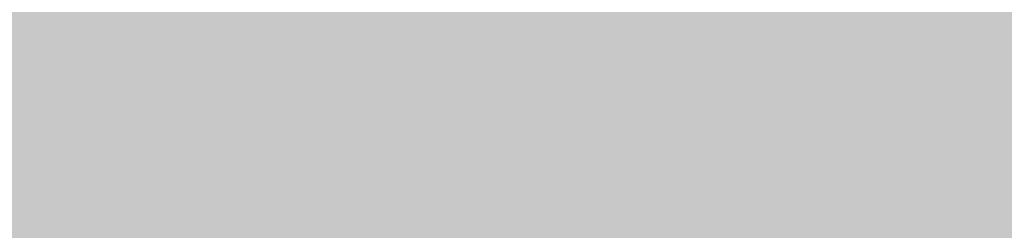
# Model space of a CAD drawing. Units: millimetres. Extents: x -22994 to 29398, y -19990 to 20176.
# Tile 73 of 135: x 226.355 to 227.437, y 83.564 to 83.796. Entities that reach past the tile are written whole.
import ezdxf
from ezdxf import colors
from ezdxf.entities.mleader import LeaderData, LeaderLine
from ezdxf.math import Vec2, Vec3

# ---------------------------------------------------------------- set-up
doc = ezdxf.new("R2010")
doc.units = ezdxf.units.MM
doc.header["$MEASUREMENT"] = 0
for name, color, linetype, lineweight in [('M-ANNO-TEXT', 7, 'Continuous', 25), ('M-DIMS', 2, 'Continuous', 18), ('M-EQPM-PATT', 7, 'Continuous', 18)]:
    doc.layers.add(name, color=color, linetype=linetype, lineweight=lineweight)
doc.styles.get("Standard").update_dxf_attribs({"font": 'arial.ttf'})
doc.dimstyles.get("Standard").update_dxf_attribs({"dimtxt": 0.18, "dimasz": 10000, "dimexe": 0.18, "dimexo": 0.0625, "dimgap": 0.09, "dimtad": 0, "dimtih": 1, "dimtoh": 1, "dimdec": 0, "dimzin": 0, "dimdsep": 46, "dimtxsty": 'Standard', "dimcen": 0.09, "dimadec": 0, "dimazin": 0, "dimtfac": 1, "dimtdec": 0, "dimtofl": 0, "dimtmove": 0, "dimatfit": 3, "dimfxl": 1, "dimtolj": 1, "dimtzin": 0, "dimlwd": 30, "dimarcsym": 0})

# ---------------------------------------------------------------- blocks, each defined once
blk = doc.blocks.new('*D2')
at = {"layer": 'Defpoints', "color": 0, "transparency": 16777216}
for p in [(6.6773, 10.2713), (290.852, 10.2713), (290.852, -5.0787)]:
    blk.add_point(p, dxfattribs=at)
at = {"layer": 'M-DIMS', "color": 0, "lineweight": -2, "transparency": 16777216}
for p, q in [((6.6773, 10.2088), (6.6773, -5.2587)), ((290.852, 10.2088), (290.852, -5.2587))]:
    blk.add_line(p, q, dxfattribs=at)
at = {"layer": 'M-DIMS', "color": 0, "lineweight": 30, "transparency": 16777216}
for p, q in [((-9993.3227, -5.0787), (-19993.3227, -5.0787)), ((10290.852, -5.0787), (20290.852, -5.0787))]:
    blk.add_line(p, q, dxfattribs=at)
at = {"layer": 'M-DIMS', "color": 0, "transparency": 16777216}
for points in [[(-9993.3227, 1661.5879), (-9993.3227, -1671.7454), (6.6773, -5.0787)], [(10290.852, 1661.5879), (10290.852, -1671.7454), (290.852, -5.0787)]]:
    blk.add_solid(points, dxfattribs=at)
at = {"layer": 'M-DIMS', "color": 0, "transparency": 16777216, "insert": (148.7647, -5.0787), "char_height": 0.18, "attachment_point": 5}
blk.add_mtext('\\A1;284.2', dxfattribs=at)
blk = doc.blocks.new('*D3')
at = {"layer": 'Defpoints', "color": 0, "transparency": 16777216}
for p in [(110.2647, 204.1654), (110.2647, 176.3662), (95.8327, 127.967)]:
    blk.add_point(p, dxfattribs=at)
at = {"layer": 'M-DIMS', "color": 0, "lineweight": -2, "transparency": 16777216}
for p, q in [((95.8327, 128.0295), (95.8327, 204.3454)), ((110.2647, 176.4287), (110.2647, 204.3454))]:
    blk.add_line(p, q, dxfattribs=at)
at = {"layer": 'M-DIMS', "color": 0, "lineweight": 30, "transparency": 16777216}
for p, q in [((-9904.1673, 204.1654), (-19904.1673, 204.1654)), ((10110.2647, 204.1654), (20110.2647, 204.1654))]:
    blk.add_line(p, q, dxfattribs=at)
at = {"layer": 'M-DIMS', "color": 0, "transparency": 16777216}
for points in [[(-9904.1673, 1870.8321), (-9904.1673, -1462.5013), (95.8327, 204.1654)], [(10110.2647, 1870.8321), (10110.2647, -1462.5013), (110.2647, 204.1654)]]:
    blk.add_solid(points, dxfattribs=at)
at = {"layer": 'M-DIMS', "color": 0, "transparency": 16777216, "insert": (103.0487, 204.1654), "char_height": 0.18, "attachment_point": 5}
blk.add_mtext('\\A1;14.432', dxfattribs=at)
blk = doc.blocks.new('*D4')
at = {"layer": 'Defpoints', "color": 0, "transparency": 16777216}
for p in [(116.2647, 204.1654), (110.2647, 176.3662), (116.2647, 176.3662)]:
    blk.add_point(p, dxfattribs=at)
at = {"layer": 'M-DIMS', "color": 0, "lineweight": -2, "transparency": 16777216}
for p, q in [((110.2647, 176.4287), (110.2647, 204.3454)), ((116.2647, 176.4287), (116.2647, 204.3454))]:
    blk.add_line(p, q, dxfattribs=at)
at = {"layer": 'M-DIMS', "color": 0, "lineweight": 30, "transparency": 16777216}
for p, q in [((-9889.7353, 204.1654), (-19889.7353, 204.1654)), ((10116.2647, 204.1654), (20116.2647, 204.1654))]:
    blk.add_line(p, q, dxfattribs=at)
at = {"layer": 'M-DIMS', "color": 0, "transparency": 16777216}
for points in [[(-9889.7353, 1870.8321), (-9889.7353, -1462.5013), (110.2647, 204.1654)], [(10116.2647, 1870.8321), (10116.2647, -1462.5013), (116.2647, 204.1654)]]:
    blk.add_solid(points, dxfattribs=at)
at = {"layer": 'M-DIMS', "color": 0, "transparency": 16777216, "insert": (113.2647, 204.1654), "char_height": 0.18, "attachment_point": 5}
blk.add_mtext('\\A1;6', dxfattribs=at)
blk = doc.blocks.new('*D5')
at = {"layer": 'Defpoints', "color": 0, "transparency": 16777216}
for p in [(181.2647, 204.1654), (116.2647, 176.3662), (181.2647, 176.3662)]:
    blk.add_point(p, dxfattribs=at)
at = {"layer": 'M-DIMS', "color": 0, "lineweight": -2, "transparency": 16777216}
for p, q in [((116.2647, 176.4287), (116.2647, 204.3454)), ((181.2647, 176.4287), (181.2647, 204.3454))]:
    blk.add_line(p, q, dxfattribs=at)
at = {"layer": 'M-DIMS', "color": 0, "lineweight": 30, "transparency": 16777216}
for p, q in [((-9883.7353, 204.1654), (-19883.7353, 204.1654)), ((10181.2647, 204.1654), (20181.2647, 204.1654))]:
    blk.add_line(p, q, dxfattribs=at)
at = {"layer": 'M-DIMS', "color": 0, "transparency": 16777216}
for points in [[(-9883.7353, 1870.8321), (-9883.7353, -1462.5013), (116.2647, 204.1654)], [(10181.2647, 1870.8321), (10181.2647, -1462.5013), (181.2647, 204.1654)]]:
    blk.add_solid(points, dxfattribs=at)
at = {"layer": 'M-DIMS', "color": 0, "transparency": 16777216, "insert": (148.7647, 204.1654), "char_height": 0.18, "attachment_point": 5}
blk.add_mtext('\\A1;65', dxfattribs=at)
blk = doc.blocks.new('*D6')
at = {"layer": 'Defpoints', "color": 0, "transparency": 16777216}
for p in [(187.2647, 204.1654), (181.2647, 176.3662), (187.2647, 176.3662)]:
    blk.add_point(p, dxfattribs=at)
at = {"layer": 'M-DIMS', "color": 0, "lineweight": -2, "transparency": 16777216}
for p, q in [((181.2647, 176.4287), (181.2647, 204.3454)), ((187.2647, 176.4287), (187.2647, 204.3454))]:
    blk.add_line(p, q, dxfattribs=at)
at = {"layer": 'M-DIMS', "color": 0, "lineweight": 30, "transparency": 16777216}
for p, q in [((-9818.7353, 204.1654), (-19818.7353, 204.1654)), ((10187.2647, 204.1654), (20187.2647, 204.1654))]:
    blk.add_line(p, q, dxfattribs=at)
at = {"layer": 'M-DIMS', "color": 0, "transparency": 16777216}
for points in [[(-9818.7353, 1870.8321), (-9818.7353, -1462.5013), (181.2647, 204.1654)], [(10187.2647, 1870.8321), (10187.2647, -1462.5013), (187.2647, 204.1654)]]:
    blk.add_solid(points, dxfattribs=at)
at = {"layer": 'M-DIMS', "color": 0, "transparency": 16777216, "insert": (184.2647, 204.1654), "char_height": 0.18, "attachment_point": 5}
blk.add_mtext('\\A1;6', dxfattribs=at)
blk = doc.blocks.new('*D7')
at = {"layer": 'Defpoints', "color": 0, "transparency": 16777216}
for p in [(201.6967, 204.1654), (187.2647, 176.3662), (201.6967, 127.967)]:
    blk.add_point(p, dxfattribs=at)
at = {"layer": 'M-DIMS', "color": 0, "lineweight": -2, "transparency": 16777216}
for p, q in [((187.2647, 176.4287), (187.2647, 204.3454)), ((201.6967, 128.0295), (201.6967, 204.3454))]:
    blk.add_line(p, q, dxfattribs=at)
at = {"layer": 'M-DIMS', "color": 0, "lineweight": 30, "transparency": 16777216}
for p, q in [((-9812.7353, 204.1654), (-19812.7353, 204.1654)), ((10201.6967, 204.1654), (20201.6967, 204.1654))]:
    blk.add_line(p, q, dxfattribs=at)
at = {"layer": 'M-DIMS', "color": 0, "transparency": 16777216}
for points in [[(-9812.7353, 1870.8321), (-9812.7353, -1462.5013), (187.2647, 204.1654)], [(10201.6967, 1870.8321), (10201.6967, -1462.5013), (201.6967, 204.1654)]]:
    blk.add_solid(points, dxfattribs=at)
at = {"layer": 'M-DIMS', "color": 0, "transparency": 16777216, "insert": (194.4807, 204.1654), "char_height": 0.18, "attachment_point": 5}
blk.add_mtext('\\A1;14.432', dxfattribs=at)
blk = doc.blocks.new('*D8')
at = {"layer": 'Defpoints', "color": 0, "transparency": 16777216}
for p in [(227.6485, 204.1654), (227.6485, 146.7296), (201.6967, 127.967)]:
    blk.add_point(p, dxfattribs=at)
at = {"layer": 'M-DIMS', "color": 0, "lineweight": -2, "transparency": 16777216}
for p, q in [((201.6967, 128.0295), (201.6967, 204.3454)), ((227.6485, 146.7921), (227.6485, 204.3454))]:
    blk.add_line(p, q, dxfattribs=at)
at = {"layer": 'M-DIMS', "color": 0, "lineweight": 30, "transparency": 16777216}
for p, q in [((-9798.3033, 204.1654), (-19798.3033, 204.1654)), ((10227.6485, 204.1654), (20227.6485, 204.1654))]:
    blk.add_line(p, q, dxfattribs=at)
at = {"layer": 'M-DIMS', "color": 0, "transparency": 16777216}
for points in [[(-9798.3033, 1870.8321), (-9798.3033, -1462.5013), (201.6967, 204.1654)], [(10227.6485, 1870.8321), (10227.6485, -1462.5013), (227.6485, 204.1654)]]:
    blk.add_solid(points, dxfattribs=at)
at = {"layer": 'M-DIMS', "color": 0, "transparency": 16777216, "insert": (214.6726, 204.1654), "char_height": 0.18, "attachment_point": 5}
blk.add_mtext('\\A1;25.95', dxfattribs=at)
blk = doc.blocks.new('*D9')
at = {"layer": 'Defpoints', "color": 0, "transparency": 16777216}
for p in [(187.2647, 176.3662), (306.202, 176.3662), (290.852, 10.2713)]:
    blk.add_point(p, dxfattribs=at)
at = {"layer": 'M-DIMS', "color": 0, "lineweight": 30, "transparency": 16777216}
for p, q in [((306.202, 10176.3662), (306.202, 20176.3662)), ((306.202, -9989.7287), (306.202, -19989.7287))]:
    blk.add_line(p, q, dxfattribs=at)
at = {"layer": 'M-DIMS', "color": 0, "lineweight": -2, "transparency": 16777216}
for p, q in [((187.3272, 176.3662), (306.382, 176.3662)), ((290.9145, 10.2713), (306.382, 10.2713))]:
    blk.add_line(p, q, dxfattribs=at)
at = {"layer": 'M-DIMS', "color": 0, "transparency": 16777216}
for points in [[(-1360.4646, 10176.3662), (1972.8687, 10176.3662), (306.202, 176.3662)], [(-1360.4646, -9989.7287), (1972.8687, -9989.7287), (306.202, 10.2713)]]:
    blk.add_solid(points, dxfattribs=at)
at = {"layer": 'M-DIMS', "color": 0, "transparency": 16777216, "insert": (306.202, 93.3187), "char_height": 0.18, "attachment_point": 5}
blk.add_mtext('\\A1;166.1', dxfattribs=at)
blk = doc.blocks.new('*D10')
at = {"layer": 'Defpoints', "color": 0, "transparency": 16777216}
for p in [(125.6498, 136.0713), (133.3459, 136.0713), (133.3459, -5.0787)]:
    blk.add_point(p, dxfattribs=at)
at = {"layer": 'M-DIMS', "color": 0, "lineweight": -2, "transparency": 16777216}
for p, q in [((125.6498, 136.0088), (125.6498, -5.2587)), ((133.3459, 136.0088), (133.3459, -5.2587))]:
    blk.add_line(p, q, dxfattribs=at)
at = {"layer": 'M-DIMS', "color": 0, "lineweight": 30, "transparency": 16777216}
for p, q in [((-9874.3502, -5.0787), (-19874.3502, -5.0787)), ((10133.3459, -5.0787), (20133.3459, -5.0787))]:
    blk.add_line(p, q, dxfattribs=at)
at = {"layer": 'M-DIMS', "color": 0, "transparency": 16777216}
for points in [[(-9874.3502, 1661.5879), (-9874.3502, -1671.7454), (125.6498, -5.0787)], [(10133.3459, 1661.5879), (10133.3459, -1671.7454), (133.3459, -5.0787)]]:
    blk.add_solid(points, dxfattribs=at)
at = {"layer": 'M-DIMS', "color": 0, "transparency": 16777216, "insert": (129.4978, -5.0787), "char_height": 0.18, "attachment_point": 5}
blk.add_mtext('\\A1;7.696', dxfattribs=at)
blk = doc.blocks.new('*D11')
at = {"layer": 'Defpoints', "color": 0, "transparency": 16777216}
for p in [(133.3459, 136.0713), (135.6498, 136.0713), (135.6498, -5.0787)]:
    blk.add_point(p, dxfattribs=at)
at = {"layer": 'M-DIMS', "color": 0, "lineweight": -2, "transparency": 16777216}
for p, q in [((133.3459, 136.0088), (133.3459, -5.2587)), ((135.6498, 136.0088), (135.6498, -5.2587))]:
    blk.add_line(p, q, dxfattribs=at)
at = {"layer": 'M-DIMS', "color": 0, "lineweight": 30, "transparency": 16777216}
for p, q in [((-9866.6541, -5.0787), (-19866.6541, -5.0787)), ((10135.6498, -5.0787), (20135.6498, -5.0787))]:
    blk.add_line(p, q, dxfattribs=at)
at = {"layer": 'M-DIMS', "color": 0, "transparency": 16777216}
for points in [[(-9866.6541, 1661.5879), (-9866.6541, -1671.7454), (133.3459, -5.0787)], [(10135.6498, 1661.5879), (10135.6498, -1671.7454), (135.6498, -5.0787)]]:
    blk.add_solid(points, dxfattribs=at)
at = {"layer": 'M-DIMS', "color": 0, "transparency": 16777216, "insert": (134.4978, -5.0787), "char_height": 0.18, "attachment_point": 5}
blk.add_mtext('\\A1;2.304', dxfattribs=at)
blk = doc.blocks.new('*D12')
at = {"layer": 'Defpoints', "color": 0, "transparency": 16777216}
for p in [(135.6498, 136.0713), (145.6498, 136.0713), (145.6498, -5.0787)]:
    blk.add_point(p, dxfattribs=at)
at = {"layer": 'M-DIMS', "color": 0, "lineweight": -2, "transparency": 16777216}
for p, q in [((135.6498, 136.0088), (135.6498, -5.2587)), ((145.6498, 136.0088), (145.6498, -5.2587))]:
    blk.add_line(p, q, dxfattribs=at)
at = {"layer": 'M-DIMS', "color": 0, "lineweight": 30, "transparency": 16777216}
for p, q in [((-9864.3502, -5.0787), (-19864.3502, -5.0787)), ((10145.6498, -5.0787), (20145.6498, -5.0787))]:
    blk.add_line(p, q, dxfattribs=at)
at = {"layer": 'M-DIMS', "color": 0, "transparency": 16777216}
for points in [[(-9864.3502, 1661.5879), (-9864.3502, -1671.7454), (135.6498, -5.0787)], [(10145.6498, 1661.5879), (10145.6498, -1671.7454), (145.6498, -5.0787)]]:
    blk.add_solid(points, dxfattribs=at)
at = {"layer": 'M-DIMS', "color": 0, "transparency": 16777216, "insert": (140.6498, -5.0787), "char_height": 0.18, "attachment_point": 5}
blk.add_mtext('\\A1;10', dxfattribs=at)
blk = doc.blocks.new('*D13')
at = {"layer": 'Defpoints', "color": 0, "transparency": 16777216}
for p in [(145.6498, 136.0713), (155.6498, 136.0713), (155.6498, -5.0787)]:
    blk.add_point(p, dxfattribs=at)
at = {"layer": 'M-DIMS', "color": 0, "lineweight": -2, "transparency": 16777216}
for p, q in [((145.6498, 136.0088), (145.6498, -5.2587)), ((155.6498, 136.0088), (155.6498, -5.2587))]:
    blk.add_line(p, q, dxfattribs=at)
at = {"layer": 'M-DIMS', "color": 0, "lineweight": 30, "transparency": 16777216}
for p, q in [((-9854.3502, -5.0787), (-19854.3502, -5.0787)), ((10155.6498, -5.0787), (20155.6498, -5.0787))]:
    blk.add_line(p, q, dxfattribs=at)
at = {"layer": 'M-DIMS', "color": 0, "transparency": 16777216}
for points in [[(-9854.3502, 1661.5879), (-9854.3502, -1671.7454), (145.6498, -5.0787)], [(10155.6498, 1661.5879), (10155.6498, -1671.7454), (155.6498, -5.0787)]]:
    blk.add_solid(points, dxfattribs=at)
at = {"layer": 'M-DIMS', "color": 0, "transparency": 16777216, "insert": (150.6498, -5.0787), "char_height": 0.18, "attachment_point": 5}
blk.add_mtext('\\A1;10', dxfattribs=at)
blk = doc.blocks.new('*D14')
at = {"layer": 'Defpoints', "color": 0, "transparency": 16777216}
for p in [(155.6498, 136.0713), (165.6498, 136.0713), (165.6498, -5.0787)]:
    blk.add_point(p, dxfattribs=at)
at = {"layer": 'M-DIMS', "color": 0, "lineweight": -2, "transparency": 16777216}
for p, q in [((155.6498, 136.0088), (155.6498, -5.2587)), ((165.6498, 136.0088), (165.6498, -5.2587))]:
    blk.add_line(p, q, dxfattribs=at)
at = {"layer": 'M-DIMS', "color": 0, "lineweight": 30, "transparency": 16777216}
for p, q in [((-9844.3502, -5.0787), (-19844.3502, -5.0787)), ((10165.6498, -5.0787), (20165.6498, -5.0787))]:
    blk.add_line(p, q, dxfattribs=at)
at = {"layer": 'M-DIMS', "color": 0, "transparency": 16777216}
for points in [[(-9844.3502, 1661.5879), (-9844.3502, -1671.7454), (155.6498, -5.0787)], [(10165.6498, 1661.5879), (10165.6498, -1671.7454), (165.6498, -5.0787)]]:
    blk.add_solid(points, dxfattribs=at)
at = {"layer": 'M-DIMS', "color": 0, "transparency": 16777216, "insert": (160.6498, -5.0787), "char_height": 0.18, "attachment_point": 5}
blk.add_mtext('\\A1;10', dxfattribs=at)
blk = doc.blocks.new('*D15')
at = {"layer": 'Defpoints', "color": 0, "transparency": 16777216}
for p in [(173.3459, 154.788), (173.3459, 136.0713), (306.202, 136.0713)]:
    blk.add_point(p, dxfattribs=at)
at = {"layer": 'M-DIMS', "color": 0, "lineweight": 30, "transparency": 16777216}
for p, q in [((306.202, 10154.788), (306.202, 20154.788)), ((306.202, -9863.9287), (306.202, -19863.9287))]:
    blk.add_line(p, q, dxfattribs=at)
at = {"layer": 'M-DIMS', "color": 0, "lineweight": -2, "transparency": 16777216}
for p, q in [((173.4084, 154.788), (306.382, 154.788)), ((173.4084, 136.0713), (306.382, 136.0713))]:
    blk.add_line(p, q, dxfattribs=at)
at = {"layer": 'M-DIMS', "color": 0, "transparency": 16777216}
for points in [[(-1360.4646, 10154.788), (1972.8687, 10154.788), (306.202, 154.788)], [(-1360.4646, -9863.9287), (1972.8687, -9863.9287), (306.202, 136.0713)]]:
    blk.add_solid(points, dxfattribs=at)
at = {"layer": 'M-DIMS', "color": 0, "transparency": 16777216, "insert": (306.202, 145.4297), "char_height": 0.18, "attachment_point": 5}
blk.add_mtext('\\A1;18.717', dxfattribs=at)
blk = doc.blocks.new('*D16')
at = {"layer": 'Defpoints', "color": 0, "transparency": 16777216}
for p in [(120.1702, 204.1654), (110.4658, 48.0349), (120.1702, 48.0349)]:
    blk.add_point(p, dxfattribs=at)
at = {"layer": 'M-DIMS', "color": 0, "lineweight": -2, "transparency": 16777216}
for p, q in [((110.4658, 48.0974), (110.4658, 204.3454)), ((120.1702, 48.0974), (120.1702, 204.3454))]:
    blk.add_line(p, q, dxfattribs=at)
at = {"layer": 'M-DIMS', "color": 0, "lineweight": 30, "transparency": 16777216}
for p, q in [((-9889.5342, 204.1654), (-19889.5342, 204.1654)), ((10120.1702, 204.1654), (20120.1702, 204.1654))]:
    blk.add_line(p, q, dxfattribs=at)
at = {"layer": 'M-DIMS', "color": 0, "transparency": 16777216}
for points in [[(-9889.5342, 1870.8321), (-9889.5342, -1462.5013), (110.4658, 204.1654)], [(10120.1702, 1870.8321), (10120.1702, -1462.5013), (120.1702, 204.1654)]]:
    blk.add_solid(points, dxfattribs=at)
at = {"layer": 'M-DIMS', "color": 0, "transparency": 16777216, "insert": (115.318, 204.1654), "char_height": 0.18, "attachment_point": 5}
blk.add_mtext('\\A1;9.704', dxfattribs=at)
blk = doc.blocks.new('*D17')
at = {"layer": 'Defpoints', "color": 0, "transparency": 16777216}
for p in [(126.1702, 204.1654), (120.1702, 48.0349), (126.1702, 48.0349)]:
    blk.add_point(p, dxfattribs=at)
at = {"layer": 'M-DIMS', "color": 0, "lineweight": -2, "transparency": 16777216}
for p, q in [((120.1702, 48.0974), (120.1702, 204.3454)), ((126.1702, 48.0974), (126.1702, 204.3454))]:
    blk.add_line(p, q, dxfattribs=at)
at = {"layer": 'M-DIMS', "color": 0, "lineweight": 30, "transparency": 16777216}
for p, q in [((-9879.8298, 204.1654), (-19879.8298, 204.1654)), ((10126.1702, 204.1654), (20126.1702, 204.1654))]:
    blk.add_line(p, q, dxfattribs=at)
at = {"layer": 'M-DIMS', "color": 0, "transparency": 16777216}
for points in [[(-9879.8298, 1870.8321), (-9879.8298, -1462.5013), (120.1702, 204.1654)], [(10126.1702, 1870.8321), (10126.1702, -1462.5013), (126.1702, 204.1654)]]:
    blk.add_solid(points, dxfattribs=at)
at = {"layer": 'M-DIMS', "color": 0, "transparency": 16777216, "insert": (123.1702, 204.1654), "char_height": 0.18, "attachment_point": 5}
blk.add_mtext('\\A1;6', dxfattribs=at)
blk = doc.blocks.new('*D18')
at = {"layer": 'Defpoints', "color": 0, "transparency": 16777216}
for p in [(132.1702, 204.1654), (126.1702, 48.0349), (132.1702, 48.0349)]:
    blk.add_point(p, dxfattribs=at)
at = {"layer": 'M-DIMS', "color": 0, "lineweight": -2, "transparency": 16777216}
for p, q in [((126.1702, 48.0974), (126.1702, 204.3454)), ((132.1702, 48.0974), (132.1702, 204.3454))]:
    blk.add_line(p, q, dxfattribs=at)
at = {"layer": 'M-DIMS', "color": 0, "lineweight": 30, "transparency": 16777216}
for p, q in [((-9873.8298, 204.1654), (-19873.8298, 204.1654)), ((10132.1702, 204.1654), (20132.1702, 204.1654))]:
    blk.add_line(p, q, dxfattribs=at)
at = {"layer": 'M-DIMS', "color": 0, "transparency": 16777216}
for points in [[(-9873.8298, 1870.8321), (-9873.8298, -1462.5013), (126.1702, 204.1654)], [(10132.1702, 1870.8321), (10132.1702, -1462.5013), (132.1702, 204.1654)]]:
    blk.add_solid(points, dxfattribs=at)
at = {"layer": 'M-DIMS', "color": 0, "transparency": 16777216, "insert": (129.1702, 204.1654), "char_height": 0.18, "attachment_point": 5}
blk.add_mtext('\\A1;6', dxfattribs=at)
blk = doc.blocks.new('*D19')
at = {"layer": 'Defpoints', "color": 0, "transparency": 16777216}
for p in [(138.1702, 204.1654), (132.1702, 48.0349), (138.1702, 48.0349)]:
    blk.add_point(p, dxfattribs=at)
at = {"layer": 'M-DIMS', "color": 0, "lineweight": -2, "transparency": 16777216}
for p, q in [((132.1702, 48.0974), (132.1702, 204.3454)), ((138.1702, 48.0974), (138.1702, 204.3454))]:
    blk.add_line(p, q, dxfattribs=at)
at = {"layer": 'M-DIMS', "color": 0, "lineweight": 30, "transparency": 16777216}
for p, q in [((-9867.8298, 204.1654), (-19867.8298, 204.1654)), ((10138.1702, 204.1654), (20138.1702, 204.1654))]:
    blk.add_line(p, q, dxfattribs=at)
at = {"layer": 'M-DIMS', "color": 0, "transparency": 16777216}
for points in [[(-9867.8298, 1870.8321), (-9867.8298, -1462.5013), (132.1702, 204.1654)], [(10138.1702, 1870.8321), (10138.1702, -1462.5013), (138.1702, 204.1654)]]:
    blk.add_solid(points, dxfattribs=at)
at = {"layer": 'M-DIMS', "color": 0, "transparency": 16777216, "insert": (135.1702, 204.1654), "char_height": 0.18, "attachment_point": 5}
blk.add_mtext('\\A1;6', dxfattribs=at)
blk = doc.blocks.new('*D20')
at = {"layer": 'Defpoints', "color": 0, "transparency": 16777216}
for p in [(144.1702, 204.1654), (138.1702, 48.0349), (144.1702, 48.0349)]:
    blk.add_point(p, dxfattribs=at)
at = {"layer": 'M-DIMS', "color": 0, "lineweight": -2, "transparency": 16777216}
for p, q in [((138.1702, 48.0974), (138.1702, 204.3454)), ((144.1702, 48.0974), (144.1702, 204.3454))]:
    blk.add_line(p, q, dxfattribs=at)
at = {"layer": 'M-DIMS', "color": 0, "lineweight": 30, "transparency": 16777216}
for p, q in [((-9861.8298, 204.1654), (-19861.8298, 204.1654)), ((10144.1702, 204.1654), (20144.1702, 204.1654))]:
    blk.add_line(p, q, dxfattribs=at)
at = {"layer": 'M-DIMS', "color": 0, "transparency": 16777216}
for points in [[(-9861.8298, 1870.8321), (-9861.8298, -1462.5013), (138.1702, 204.1654)], [(10144.1702, 1870.8321), (10144.1702, -1462.5013), (144.1702, 204.1654)]]:
    blk.add_solid(points, dxfattribs=at)
at = {"layer": 'M-DIMS', "color": 0, "transparency": 16777216, "insert": (141.1702, 204.1654), "char_height": 0.18, "attachment_point": 5}
blk.add_mtext('\\A1;6', dxfattribs=at)
blk = doc.blocks.new('*D21')
at = {"layer": 'Defpoints', "color": 0, "transparency": 16777216}
for p in [(149.1157, 204.1654), (144.1702, 48.0349), (149.1157, 48.0349)]:
    blk.add_point(p, dxfattribs=at)
at = {"layer": 'M-DIMS', "color": 0, "lineweight": -2, "transparency": 16777216}
for p, q in [((144.1702, 48.0974), (144.1702, 204.3454)), ((149.1157, 48.0974), (149.1157, 204.3454))]:
    blk.add_line(p, q, dxfattribs=at)
at = {"layer": 'M-DIMS', "color": 0, "lineweight": 30, "transparency": 16777216}
for p, q in [((-9855.8298, 204.1654), (-19855.8298, 204.1654)), ((10149.1157, 204.1654), (20149.1157, 204.1654))]:
    blk.add_line(p, q, dxfattribs=at)
at = {"layer": 'M-DIMS', "color": 0, "transparency": 16777216}
for points in [[(-9855.8298, 1870.8321), (-9855.8298, -1462.5013), (144.1702, 204.1654)], [(10149.1157, 1870.8321), (10149.1157, -1462.5013), (149.1157, 204.1654)]]:
    blk.add_solid(points, dxfattribs=at)
at = {"layer": 'M-DIMS', "color": 0, "transparency": 16777216, "insert": (146.6429, 204.1654), "char_height": 0.18, "attachment_point": 5}
blk.add_mtext('\\A1;4.945', dxfattribs=at)
blk = doc.blocks.new('*D22')
at = {"layer": 'Defpoints', "color": 0, "transparency": 16777216}
for p in [(149.1157, 30.9895), (155.1157, 30.9895), (155.1157, -5.0787)]:
    blk.add_point(p, dxfattribs=at)
at = {"layer": 'M-DIMS', "color": 0, "lineweight": -2, "transparency": 16777216}
for p, q in [((149.1157, 30.927), (149.1157, -5.2587)), ((155.1157, 30.927), (155.1157, -5.2587))]:
    blk.add_line(p, q, dxfattribs=at)
at = {"layer": 'M-DIMS', "color": 0, "lineweight": 30, "transparency": 16777216}
for p, q in [((-9850.8843, -5.0787), (-19850.8843, -5.0787)), ((10155.1157, -5.0787), (20155.1157, -5.0787))]:
    blk.add_line(p, q, dxfattribs=at)
at = {"layer": 'M-DIMS', "color": 0, "transparency": 16777216}
for points in [[(-9850.8843, 1661.5879), (-9850.8843, -1671.7454), (149.1157, -5.0787)], [(10155.1157, 1661.5879), (10155.1157, -1671.7454), (155.1157, -5.0787)]]:
    blk.add_solid(points, dxfattribs=at)
at = {"layer": 'M-DIMS', "color": 0, "transparency": 16777216, "insert": (152.1157, -5.0787), "char_height": 0.18, "attachment_point": 5}
blk.add_mtext('\\A1;6', dxfattribs=at)
blk = doc.blocks.new('*D23')
at = {"layer": 'Defpoints', "color": 0, "transparency": 16777216}
for p in [(155.1157, 30.9895), (161.1157, 30.9895), (161.1157, -5.0787)]:
    blk.add_point(p, dxfattribs=at)
at = {"layer": 'M-DIMS', "color": 0, "lineweight": -2, "transparency": 16777216}
for p, q in [((155.1157, 30.927), (155.1157, -5.2587)), ((161.1157, 30.927), (161.1157, -5.2587))]:
    blk.add_line(p, q, dxfattribs=at)
at = {"layer": 'M-DIMS', "color": 0, "lineweight": 30, "transparency": 16777216}
for p, q in [((-9844.8843, -5.0787), (-19844.8843, -5.0787)), ((10161.1157, -5.0787), (20161.1157, -5.0787))]:
    blk.add_line(p, q, dxfattribs=at)
at = {"layer": 'M-DIMS', "color": 0, "transparency": 16777216}
for points in [[(-9844.8843, 1661.5879), (-9844.8843, -1671.7454), (155.1157, -5.0787)], [(10161.1157, 1661.5879), (10161.1157, -1671.7454), (161.1157, -5.0787)]]:
    blk.add_solid(points, dxfattribs=at)
at = {"layer": 'M-DIMS', "color": 0, "transparency": 16777216, "insert": (158.1157, -5.0787), "char_height": 0.18, "attachment_point": 5}
blk.add_mtext('\\A1;6', dxfattribs=at)
blk = doc.blocks.new('*D24')
at = {"layer": 'Defpoints', "color": 0, "transparency": 16777216}
for p in [(161.1157, 30.9895), (166.4387, 30.9895), (166.4387, -5.0787)]:
    blk.add_point(p, dxfattribs=at)
at = {"layer": 'M-DIMS', "color": 0, "lineweight": -2, "transparency": 16777216}
for p, q in [((161.1157, 30.927), (161.1157, -5.2587)), ((166.4387, 30.927), (166.4387, -5.2587))]:
    blk.add_line(p, q, dxfattribs=at)
at = {"layer": 'M-DIMS', "color": 0, "lineweight": 30, "transparency": 16777216}
for p, q in [((-9838.8843, -5.0787), (-19838.8843, -5.0787)), ((10166.4387, -5.0787), (20166.4387, -5.0787))]:
    blk.add_line(p, q, dxfattribs=at)
at = {"layer": 'M-DIMS', "color": 0, "transparency": 16777216}
for points in [[(-9838.8843, 1661.5879), (-9838.8843, -1671.7454), (161.1157, -5.0787)], [(10166.4387, 1661.5879), (10166.4387, -1671.7454), (166.4387, -5.0787)]]:
    blk.add_solid(points, dxfattribs=at)
at = {"layer": 'M-DIMS', "color": 0, "transparency": 16777216, "insert": (163.7772, -5.0787), "char_height": 0.18, "attachment_point": 5}
blk.add_mtext('\\A1;5.323', dxfattribs=at)
blk = doc.blocks.new('*D25')
at = {"layer": 'Defpoints', "color": 0, "transparency": 16777216}
for p in [(166.4387, 30.9895), (172.4387, 30.9895), (172.4387, -5.0787)]:
    blk.add_point(p, dxfattribs=at)
at = {"layer": 'M-DIMS', "color": 0, "lineweight": -2, "transparency": 16777216}
for p, q in [((166.4387, 30.927), (166.4387, -5.2587)), ((172.4387, 30.927), (172.4387, -5.2587))]:
    blk.add_line(p, q, dxfattribs=at)
at = {"layer": 'M-DIMS', "color": 0, "lineweight": 30, "transparency": 16777216}
for p, q in [((-9833.5613, -5.0787), (-19833.5613, -5.0787)), ((10172.4387, -5.0787), (20172.4387, -5.0787))]:
    blk.add_line(p, q, dxfattribs=at)
at = {"layer": 'M-DIMS', "color": 0, "transparency": 16777216}
for points in [[(-9833.5613, 1661.5879), (-9833.5613, -1671.7454), (166.4387, -5.0787)], [(10172.4387, 1661.5879), (10172.4387, -1671.7454), (172.4387, -5.0787)]]:
    blk.add_solid(points, dxfattribs=at)
at = {"layer": 'M-DIMS', "color": 0, "transparency": 16777216, "insert": (169.4387, -5.0787), "char_height": 0.18, "attachment_point": 5}
blk.add_mtext('\\A1;6', dxfattribs=at)
blk = doc.blocks.new('*D26')
at = {"layer": 'Defpoints', "color": 0, "transparency": 16777216}
for p in [(172.4387, 30.9895), (178.4387, 30.9895), (178.4387, -5.0787)]:
    blk.add_point(p, dxfattribs=at)
at = {"layer": 'M-DIMS', "color": 0, "lineweight": -2, "transparency": 16777216}
for p, q in [((172.4387, 30.927), (172.4387, -5.2587)), ((178.4387, 30.927), (178.4387, -5.2587))]:
    blk.add_line(p, q, dxfattribs=at)
at = {"layer": 'M-DIMS', "color": 0, "lineweight": 30, "transparency": 16777216}
for p, q in [((-9827.5613, -5.0787), (-19827.5613, -5.0787)), ((10178.4387, -5.0787), (20178.4387, -5.0787))]:
    blk.add_line(p, q, dxfattribs=at)
at = {"layer": 'M-DIMS', "color": 0, "transparency": 16777216}
for points in [[(-9827.5613, 1661.5879), (-9827.5613, -1671.7454), (172.4387, -5.0787)], [(10178.4387, 1661.5879), (10178.4387, -1671.7454), (178.4387, -5.0787)]]:
    blk.add_solid(points, dxfattribs=at)
at = {"layer": 'M-DIMS', "color": 0, "transparency": 16777216, "insert": (175.4387, -5.0787), "char_height": 0.18, "attachment_point": 5}
blk.add_mtext('\\A1;6', dxfattribs=at)
blk = doc.blocks.new('*D27')
at = {"layer": 'Defpoints', "color": 0, "transparency": 16777216}
for p in [(178.4387, 30.9895), (188.1175, 30.9895), (188.1175, -5.0787)]:
    blk.add_point(p, dxfattribs=at)
at = {"layer": 'M-DIMS', "color": 0, "lineweight": -2, "transparency": 16777216}
for p, q in [((178.4387, 30.927), (178.4387, -5.2587)), ((188.1175, 30.927), (188.1175, -5.2587))]:
    blk.add_line(p, q, dxfattribs=at)
at = {"layer": 'M-DIMS', "color": 0, "lineweight": 30, "transparency": 16777216}
for p, q in [((-9821.5613, -5.0787), (-19821.5613, -5.0787)), ((10188.1175, -5.0787), (20188.1175, -5.0787))]:
    blk.add_line(p, q, dxfattribs=at)
at = {"layer": 'M-DIMS', "color": 0, "transparency": 16777216}
for points in [[(-9821.5613, 1661.5879), (-9821.5613, -1671.7454), (178.4387, -5.0787)], [(10188.1175, 1661.5879), (10188.1175, -1671.7454), (188.1175, -5.0787)]]:
    blk.add_solid(points, dxfattribs=at)
at = {"layer": 'M-DIMS', "color": 0, "transparency": 16777216, "insert": (183.2781, -5.0787), "char_height": 0.18, "attachment_point": 5}
blk.add_mtext('\\A1;9.679', dxfattribs=at)
blk = doc.blocks.new('*D28')
at = {"layer": 'Defpoints', "color": 0, "transparency": 16777216}
for p in [(188.1175, 48.0349), (306.202, 48.0349), (188.1175, 30.9895)]:
    blk.add_point(p, dxfattribs=at)
at = {"layer": 'M-DIMS', "color": 0, "lineweight": 30, "transparency": 16777216}
for p, q in [((306.202, 10048.0349), (306.202, 20048.0349)), ((306.202, -9969.0105), (306.202, -19969.0105))]:
    blk.add_line(p, q, dxfattribs=at)
at = {"layer": 'M-DIMS', "color": 0, "lineweight": -2, "transparency": 16777216}
for p, q in [((188.18, 48.0349), (306.382, 48.0349)), ((188.18, 30.9895), (306.382, 30.9895))]:
    blk.add_line(p, q, dxfattribs=at)
at = {"layer": 'M-DIMS', "color": 0, "transparency": 16777216}
for points in [[(-1360.4646, 10048.0349), (1972.8687, 10048.0349), (306.202, 48.0349)], [(-1360.4646, -9969.0105), (1972.8687, -9969.0105), (306.202, 30.9895)]]:
    blk.add_solid(points, dxfattribs=at)
at = {"layer": 'M-DIMS', "color": 0, "transparency": 16777216, "insert": (306.202, 39.5122), "char_height": 0.18, "attachment_point": 5}
blk.add_mtext('\\A1;17.045', dxfattribs=at)
blk = doc.blocks.new('*D29')
at = {"layer": 'Defpoints', "color": 0, "transparency": 16777216}
for p in [(36.8006, 80.045), (64.0296, 80.045)]:
    blk.add_point(p, dxfattribs=at)
at = {"layer": 'M-DIMS', "color": 0, "lineweight": -2, "transparency": 16777216}
for p, q in [((50.4151, 79.955), (50.4151, 80.135)), ((50.3251, 80.045), (50.5051, 80.045))]:
    blk.add_line(p, q, dxfattribs=at)
at = {"layer": 'M-DIMS', "color": 0, "lineweight": 30, "transparency": 16777216}
blk.add_line((20064.0296, 80.0303), (10064.0296, 80.0377), dxfattribs=at)
at = {"layer": 'M-DIMS', "color": 0, "transparency": 16777216}
blk.add_solid([(10064.0309, 1746.7043), (10064.0284, -1586.629), (64.0296, 80.045)], dxfattribs=at)
at = {"layer": 'M-DIMS', "color": 0, "transparency": 16777216, "insert": (20064.5213, 80.0303), "char_height": 0.18, "attachment_point": 5}
blk.add_mtext('\\A1;∅27.23', dxfattribs=at)
blk = doc.blocks.new('*D30')
at = {"layer": 'Defpoints', "color": 0, "transparency": 16777216}
for p in [(216.3148, 146.7291), (238.9821, 146.73)]:
    blk.add_point(p, dxfattribs=at)
at = {"layer": 'M-DIMS', "color": 0, "lineweight": 30, "transparency": 16777216}
blk.add_line((20238.9821, 147.4959), (10238.9821, 147.1129), dxfattribs=at)
at = {"layer": 'M-DIMS', "color": 0, "lineweight": -2, "transparency": 16777216}
for p, q in [((227.6485, 146.6396), (227.6485, 146.8196)), ((227.5585, 146.7296), (227.7385, 146.7296))]:
    blk.add_line(p, q, dxfattribs=at)
at = {"layer": 'M-DIMS', "color": 0, "transparency": 16777216}
blk.add_solid([(10238.9183, 1813.7796), (10239.0459, -1519.5537), (238.9821, 146.73)], dxfattribs=at)
at = {"layer": 'M-DIMS', "color": 0, "transparency": 16777216, "insert": (20239.5436, 147.4959), "char_height": 0.18, "attachment_point": 5}
blk.add_mtext('\\A1;∅22.667', dxfattribs=at)
blk = doc.blocks.new('*D31')
at = {"layer": 'Defpoints', "color": 0, "transparency": 16777216}
for p in [(223.1641, 146.7291), (232.1328, 146.73)]:
    blk.add_point(p, dxfattribs=at)
at = {"layer": 'M-DIMS', "color": 0, "lineweight": 30, "transparency": 16777216}
blk.add_line((20232.1327, 148.6656), (10232.1328, 147.6978), dxfattribs=at)
at = {"layer": 'M-DIMS', "color": 0, "lineweight": -2, "transparency": 16777216}
for p, q in [((227.6485, 146.6396), (227.6485, 146.8196)), ((227.5585, 146.7296), (227.7385, 146.7296))]:
    blk.add_line(p, q, dxfattribs=at)
at = {"layer": 'M-DIMS', "color": 0, "transparency": 16777216}
blk.add_solid([(10231.9715, 1814.3645), (10232.2941, -1518.9688), (232.1328, 146.73)], dxfattribs=at)
at = {"layer": 'M-DIMS', "color": 0, "transparency": 16777216, "insert": (20232.6245, 148.6656), "char_height": 0.18, "attachment_point": 5}
blk.add_mtext('\\A1;∅8.969', dxfattribs=at)
blk = doc.blocks.new('*D36')
at = {"layer": 'Defpoints', "color": 0, "transparency": 16777216}
for p in [(46.39, 31.3035), (46.3875, 26.5934)]:
    blk.add_point(p, dxfattribs=at)
at = {"layer": 'M-DIMS', "color": 0, "lineweight": 30, "transparency": 16777216}
for p, q in [((57.1499, 20031.3006), (51.77, 10031.302)), ((10057.1499, 20031.3006), (57.1499, 20031.3006))]:
    blk.add_line(p, q, dxfattribs=at)
at = {"layer": 'M-DIMS', "color": 0, "lineweight": -2, "transparency": 16777216}
for p, q in [((46.3887, 28.8585), (46.3887, 29.0385)), ((46.2987, 28.9485), (46.4787, 28.9485))]:
    blk.add_line(p, q, dxfattribs=at)
at = {"layer": 'M-DIMS', "color": 0, "transparency": 16777216}
blk.add_solid([(-1614.8965, 10032.1987), (1718.4364, 10030.4054), (46.39, 31.3035)], dxfattribs=at)
at = {"layer": 'M-DIMS', "color": 0, "transparency": 16777216, "insert": (10057.5542, 20031.3006), "char_height": 0.18, "attachment_point": 5}
blk.add_mtext('\\A1;∅4.71', dxfattribs=at)
blk = doc.blocks.new('*D37')
at = {"layer": 'Defpoints', "color": 0, "transparency": 16777216}
for p in [(54.8343, 118.6145), (59.4936, 118.614)]:
    blk.add_point(p, dxfattribs=at)
at = {"layer": 'M-DIMS', "color": 0, "lineweight": -2, "transparency": 16777216}
for p, q in [((57.1639, 118.5243), (57.1639, 118.7043)), ((57.0739, 118.6143), (57.2539, 118.6143))]:
    blk.add_line(p, q, dxfattribs=at)
at = {"layer": 'M-DIMS', "color": 0, "lineweight": 30, "transparency": 16777216}
blk.add_line((20059.4934, 116.2531), (10059.4935, 117.4336), dxfattribs=at)
at = {"layer": 'M-DIMS', "color": 0, "transparency": 16777216}
blk.add_solid([(10059.6902, 1784.1002), (10059.2968, -1549.2331), (59.4936, 118.614)], dxfattribs=at)
at = {"layer": 'M-DIMS', "color": 0, "transparency": 16777216, "insert": (20059.9852, 116.2531), "char_height": 0.18, "attachment_point": 5}
blk.add_mtext('\\A1;∅4.659', dxfattribs=at)

msp = doc.modelspace()

# ---------------------------------------------------------------- hatches: boundary and pattern name
at = {"layer": 'M-EQPM-PATT'}
h = msp.add_hatch(color=256, dxfattribs=at)
h.set_gradient(color1=(205, 32, 39), color2=(205, 32, 39), tint=1)
h.paths.add_polyline_path([(116.2647, 150.3662), (116.2647, 170.3662), (116.2647, 176.3662), (110.2647, 176.3662), (110.2647, 152.0276), (95.8327, 127.967), (95.8327, 16.6063), (201.6967, 16.6063), (201.6967, 127.967), (187.2647, 152.0276), (187.2647, 176.3662), (181.2647, 176.3662), (181.2647, 170.3662), (181.2647, 150.3662), (195.6967, 126.3055), (195.6967, 22.6063), (101.8327, 22.6063), (101.8327, 126.3055)])
h.paths.add_polyline_path([(185.2208, 88.6347), (101.8327, 88.6347), (101.8327, 87.6347), (182.8066, 87.6347), (178.7313, 83.5594), (195.6967, 83.5594), (195.6967, 84.5594), (181.1455, 84.5594)], flags=17)
h.paths.add_polyline_path([(95.8327, 88.6347), (60.9779, 88.6347, -0.022855), (61.7178, 87.6347), (95.8327, 87.6347)])
h.paths.add_polyline_path([(215.6212, 86.5189), (215.6212, 80.5999), (220.5095, 83.5594)])
h.paths.add_polyline_path([(215.6212, 84.5594), (201.6967, 84.5594), (201.6967, 83.5594), (215.6212, 83.5594)])
h.paths.add_polyline_path([(225.3978, 86.5189), (220.5095, 83.5594), (225.3978, 80.5999)])
h.paths.add_polyline_path([(231.6256, 84.5594), (225.3978, 84.5594), (225.3978, 83.5594), (231.6256, 83.5594)])

# ---------------------------------------------------------------- dimensions: what is measured, and where the dimension line sits
at = {"layer": 'M-DIMS'}
for base, p1, p2, override, picture, middle in [((306.202, 176.3662), (290.852, 10.2713), (187.2647, 176.3662), {"dimdec": 1, "dimlfac": 1, "dimrnd": 0, "dimzin": 0, "dimdsep": 46, "dimlunit": 2}, '*D9', (306.202, 93.3187)), ((306.202, 136.0713), (173.3459, 154.788), (173.3459, 136.0713), {"dimdec": 3, "dimlfac": 1, "dimrnd": 0, "dimzin": 0, "dimdsep": 46, "dimlunit": 2}, '*D15', (306.202, 145.4297)), ((306.202, 48.0349), (188.1175, 30.9895), (188.1175, 48.0349), {"dimdec": 3, "dimlfac": 1, "dimrnd": 0, "dimzin": 0, "dimdsep": 46, "dimlunit": 2}, '*D28', (306.202, 39.5122))]:
    dim = msp.add_linear_dim(base=base, p1=p1, p2=p2, angle=90, dimstyle='Standard', override=override, dxfattribs=at)
    dim.commit()
    dim.dimension.update_dxf_attribs({"geometry": picture, "text_midpoint": middle})
for p1, p2, override, picture, middle in [((46.3875, 26.5934), (46.39, 31.3035), {"dimdec": 2, "dimlfac": 1, "dimrnd": 0, "dimzin": 0, "dimdsep": 46, "dimlunit": 2}, '*D36', (10057.5542, 20031.3006)), ((223.1641, 146.7291), (232.1328, 146.73), {"dimdec": 3, "dimlfac": 1, "dimrnd": 0, "dimzin": 0, "dimdsep": 46, "dimlunit": 2}, '*D31', (20232.1327, 148.6656)), ((216.3148, 146.7291), (238.9821, 146.73), {"dimdec": 3, "dimlfac": 1, "dimrnd": 0, "dimzin": 0, "dimdsep": 46, "dimlunit": 2}, '*D30', (20238.9821, 147.4959))]:
    dim = msp.add_diameter_dim_2p(p1=p1, p2=p2, dimstyle='Standard', override=override, dxfattribs=at)
    dim.commit()
    dim.dimension.update_dxf_attribs({"geometry": picture, "text_midpoint": middle, "dimtype": 163})
for base, p1, p2, override, picture, middle in [((110.2647, 204.1654), (95.8327, 127.967), (110.2647, 176.3662), {"dimdec": 3, "dimlfac": 1, "dimrnd": 0, "dimzin": 0, "dimdsep": 46, "dimlunit": 2}, '*D3', (103.0487, 204.1654)), ((116.2647, 204.1654), (110.2647, 176.3662), (116.2647, 176.3662), {"dimdec": 0, "dimlfac": 1, "dimrnd": 0, "dimzin": 0, "dimdsep": 46, "dimlunit": 2}, '*D4', (113.2647, 204.1654)), ((120.1702, 204.1654), (110.4658, 48.0349), (120.1702, 48.0349), {"dimdec": 3, "dimlfac": 1, "dimrnd": 0, "dimzin": 0, "dimdsep": 46, "dimlunit": 2}, '*D16', (115.318, 204.1654)), ((181.2647, 204.1654), (116.2647, 176.3662), (181.2647, 176.3662), {"dimdec": 0, "dimlfac": 1, "dimrnd": 0, "dimzin": 0, "dimdsep": 46, "dimlunit": 2}, '*D5', (148.7647, 204.1654)), ((126.1702, 204.1654), (120.1702, 48.0349), (126.1702, 48.0349), {"dimdec": 0, "dimlfac": 1, "dimrnd": 0, "dimzin": 0, "dimdsep": 46, "dimlunit": 2}, '*D17', (123.1702, 204.1654)), ((132.1702, 204.1654), (126.1702, 48.0349), (132.1702, 48.0349), {"dimdec": 0, "dimlfac": 1, "dimrnd": 0, "dimzin": 0, "dimdsep": 46, "dimlunit": 2}, '*D18', (129.1702, 204.1654)), ((138.1702, 204.1654), (132.1702, 48.0349), (138.1702, 48.0349), {"dimdec": 0, "dimlfac": 1, "dimrnd": 0, "dimzin": 0, "dimdsep": 46, "dimlunit": 2}, '*D19', (135.1702, 204.1654)), ((144.1702, 204.1654), (138.1702, 48.0349), (144.1702, 48.0349), {"dimdec": 0, "dimlfac": 1, "dimrnd": 0, "dimzin": 0, "dimdsep": 46, "dimlunit": 2}, '*D20', (141.1702, 204.1654)), ((149.11567, 204.16539), (144.17023, 48.03494), (149.11567, 48.03494), {"dimdec": 3, "dimlfac": 1, "dimrnd": 0, "dimzin": 0, "dimdsep": 46, "dimlunit": 2}, '*D21', (146.64295, 204.16539)), ((187.2647, 204.1654), (181.2647, 176.3662), (187.2647, 176.3662), {"dimdec": 0, "dimlfac": 1, "dimrnd": 0, "dimzin": 0, "dimdsep": 46, "dimlunit": 2}, '*D6', (184.2647, 204.1654)), ((201.6967, 204.1654), (187.2647, 176.3662), (201.6967, 127.967), {"dimdec": 3, "dimlfac": 1, "dimrnd": 0, "dimzin": 0, "dimdsep": 46, "dimlunit": 2}, '*D7', (194.4807, 204.1654)), ((227.6485, 204.1654), (201.6967, 127.967), (227.6485, 146.7296), {"dimdec": 2, "dimlfac": 1, "dimrnd": 0, "dimzin": 0, "dimdsep": 46, "dimlunit": 2}, '*D8', (214.6726, 204.1654)), ((290.852, -5.0787), (6.6773, 10.2713), (290.852, 10.2713), {"dimdec": 1, "dimlfac": 1, "dimrnd": 0, "dimzin": 0, "dimdsep": 46, "dimlunit": 2}, '*D2', (148.7647, -5.0787)), ((133.3459, -5.0787), (125.6498, 136.0713), (133.3459, 136.0713), {"dimdec": 3, "dimlfac": 1, "dimrnd": 0, "dimzin": 0, "dimdsep": 46, "dimlunit": 2}, '*D10', (129.4978, -5.0787)), ((135.6498, -5.0787), (133.3459, 136.0713), (135.6498, 136.0713), {"dimdec": 3, "dimlfac": 1, "dimrnd": 0, "dimzin": 0, "dimdsep": 46, "dimlunit": 2}, '*D11', (134.4978, -5.0787)), ((145.6498, -5.0787), (135.6498, 136.0713), (145.6498, 136.0713), {"dimdec": 0, "dimlfac": 1, "dimrnd": 0, "dimzin": 0, "dimdsep": 46, "dimlunit": 2}, '*D12', (140.6498, -5.0787)), ((155.6498, -5.0787), (145.6498, 136.0713), (155.6498, 136.0713), {"dimdec": 0, "dimlfac": 1, "dimrnd": 0, "dimzin": 0, "dimdsep": 46, "dimlunit": 2}, '*D13', (150.6498, -5.0787)), ((155.1157, -5.0787), (149.1157, 30.9895), (155.1157, 30.9895), {"dimdec": 0, "dimlfac": 1, "dimrnd": 0, "dimzin": 0, "dimdsep": 46, "dimlunit": 2}, '*D22', (152.1157, -5.0787)), ((161.1157, -5.0787), (155.1157, 30.9895), (161.1157, 30.9895), {"dimdec": 0, "dimlfac": 1, "dimrnd": 0, "dimzin": 0, "dimdsep": 46, "dimlunit": 2}, '*D23', (158.1157, -5.0787)), ((165.6498, -5.0787), (155.6498, 136.0713), (165.6498, 136.0713), {"dimdec": 0, "dimlfac": 1, "dimrnd": 0, "dimzin": 0, "dimdsep": 46, "dimlunit": 2}, '*D14', (160.6498, -5.0787)), ((166.4387, -5.0787), (161.1157, 30.9895), (166.4387, 30.9895), {"dimdec": 3, "dimlfac": 1, "dimrnd": 0, "dimzin": 0, "dimdsep": 46, "dimlunit": 2}, '*D24', (163.7772, -5.0787)), ((172.4387, -5.0787), (166.4387, 30.9895), (172.4387, 30.9895), {"dimdec": 0, "dimlfac": 1, "dimrnd": 0, "dimzin": 0, "dimdsep": 46, "dimlunit": 2}, '*D25', (169.4387, -5.0787)), ((178.4387, -5.0787), (172.4387, 30.9895), (178.4387, 30.9895), {"dimdec": 0, "dimlfac": 1, "dimrnd": 0, "dimzin": 0, "dimdsep": 46, "dimlunit": 2}, '*D26', (175.4387, -5.0787)), ((188.1175, -5.0787), (178.4387, 30.9895), (188.1175, 30.9895), {"dimdec": 3, "dimlfac": 1, "dimrnd": 0, "dimzin": 0, "dimdsep": 46, "dimlunit": 2}, '*D27', (183.2781, -5.0787))]:
    dim = msp.add_linear_dim(base=base, p1=p1, p2=p2, dimstyle='Standard', override=override, dxfattribs=at)
    dim.commit()
    dim.dimension.update_dxf_attribs({"geometry": picture, "text_midpoint": middle})
for p1, p2, override, picture, middle in [((54.8343, 118.6145), (59.4936, 118.614), {"dimdec": 3, "dimlfac": 1, "dimrnd": 0, "dimzin": 0, "dimdsep": 46, "dimlunit": 2}, '*D37', (20059.4934, 116.2531)), ((36.8006, 80.045), (64.0296, 80.045), {"dimdec": 2, "dimlfac": 1, "dimrnd": 0, "dimzin": 0, "dimdsep": 46, "dimlunit": 2}, '*D29', (20064.0296, 80.0303))]:
    dim = msp.add_diameter_dim_2p(p1=p1, p2=p2, dimstyle='Standard', override=override, dxfattribs=at)
    dim.commit()
    dim.dimension.update_dxf_attribs({"geometry": picture, "text_midpoint": middle})

# ---------------------------------------------------------------- leaders
at = {"layer": 'M-ANNO-TEXT'}
ml = msp.add_multileader_mtext('Standard', dxfattribs=at)
ml.set_content('combustion chamber', color=256)
ml.set_leader_properties()
ml.build(insert=Vec2(0, 0))
ml.multileader.update_dxf_attribs({"dogleg_length": 0.36, "arrow_head_size": 200})
ctx = ml.context
ctx.base_point, ctx.char_height, ctx.arrow_head_size, ctx.landing_gap_size, ctx.plane_origin = Vec3(215.7321, 57.9149), 3, 200, 0.09, Vec3(189.1175, 57.9149)
notes = []
notes.append((ctx, [(0, (1, 1, 0), (215.3721, 57.9149), (1, 0), 0.36, [(0, [(189.1175, 57.9149)], 0, [])])]))
ctx.mtext.insert, ctx.mtext.flow_direction = Vec3(215.8221, 59.4394), 5
for ctx, leaders in notes:
    for number, flags, end, landing, length, lines in leaders:
        leader = LeaderData()
        leader.index, (leader.has_last_leader_line, leader.has_dogleg_vector, leader.attachment_direction) = number, flags
        leader.last_leader_point, leader.dogleg_vector, leader.dogleg_length = Vec3(end), Vec3(landing), length
        for number, points, colour, breaks in lines:
            line = LeaderLine()
            line.index, line.vertices, line.color, line.breaks = number, Vec3.list(points), colors.encode_raw_color(colour), breaks
            leader.lines.append(line)
        ctx.leaders.append(leader)

doc.saveas('drawing.dxf')
